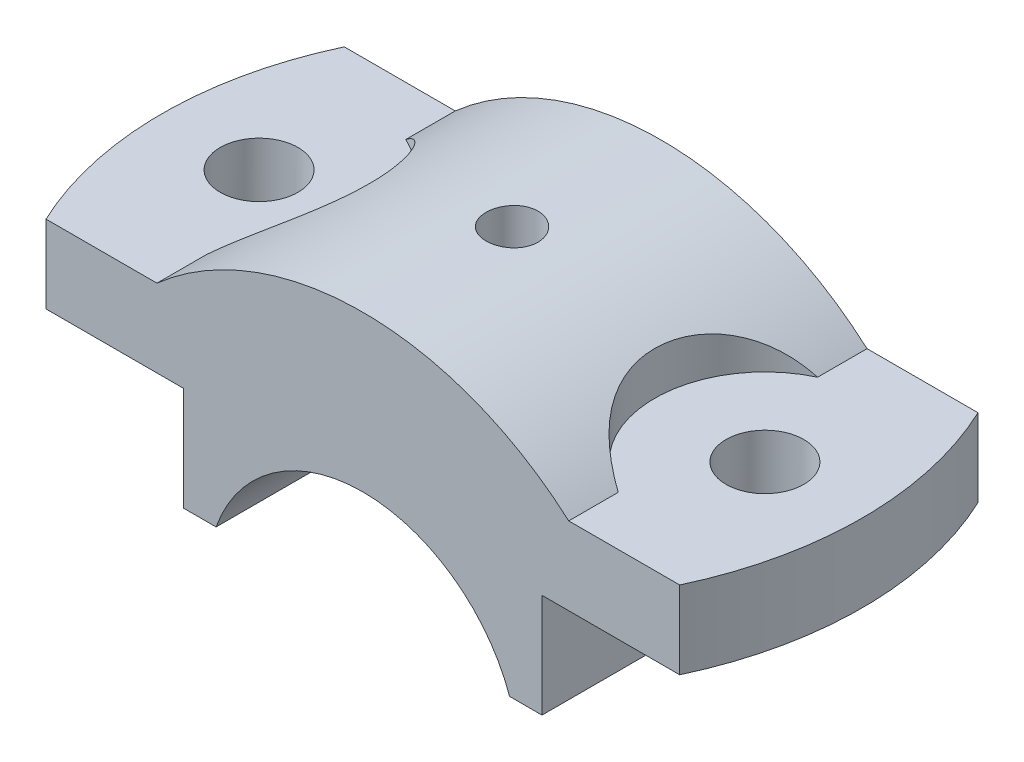
ISO-10303-21;
HEADER;
FILE_DESCRIPTION(('STEP AP214'),'2;1');
FILE_NAME('part.step','',(''),(''),'','','');
FILE_SCHEMA(('AUTOMOTIVE_DESIGN { 1 0 10303 214 1 1 1 1 }'));
ENDSEC;
DATA;
#1=APPLICATION_CONTEXT('core data for automotive mechanical design processes');
#2=APPLICATION_PROTOCOL_DEFINITION('international standard','automotive_design',2000,#1);
#3=PRODUCT_CONTEXT('',#1,'mechanical');
#4=PRODUCT('Part','Part','',(#3));
#5=PRODUCT_RELATED_PRODUCT_CATEGORY('part','',(#4));
#6=PRODUCT_DEFINITION_FORMATION('','',#4);
#7=PRODUCT_DEFINITION_CONTEXT('part definition',#1,'design');
#8=PRODUCT_DEFINITION('design','',#6,#7);
#9=PRODUCT_DEFINITION_SHAPE('','',#8);
#10=(LENGTH_UNIT() NAMED_UNIT(*) SI_UNIT(.MILLI.,.METRE.));
#11=(NAMED_UNIT(*) PLANE_ANGLE_UNIT() SI_UNIT($,.RADIAN.));
#12=(NAMED_UNIT(*) SI_UNIT($,.STERADIAN.) SOLID_ANGLE_UNIT());
#13=UNCERTAINTY_MEASURE_WITH_UNIT(LENGTH_MEASURE(1.E-05),#10,'distance_accuracy_value','');
#14=(GEOMETRIC_REPRESENTATION_CONTEXT(3) GLOBAL_UNCERTAINTY_ASSIGNED_CONTEXT((#13)) GLOBAL_UNIT_ASSIGNED_CONTEXT((#10,
#11,#12)) REPRESENTATION_CONTEXT('',''));
#15=CARTESIAN_POINT('',(0.,0.,0.));
#16=DIRECTION('',(0.,0.,1.));
#17=DIRECTION('',(1.,0.,0.));
#18=AXIS2_PLACEMENT_3D('',#15,#16,#17);
#19=CARTESIAN_POINT('',(27.6274169979695,24.,23.));
#20=DIRECTION('',(0.,1.,0.));
#21=DIRECTION('',(-1.,0.,0.));
#22=AXIS2_PLACEMENT_3D('',#19,#20,#21);
#23=PLANE('',#22);
#24=CARTESIAN_POINT('',(39.,24.,0.));
#25=DIRECTION('',(0.,1.,0.));
#26=DIRECTION('',(-1.,0.,0.));
#27=AXIS2_PLACEMENT_3D('',#24,#25,#26);
#28=CIRCLE('',#27,5.99999999999999);
#29=CARTESIAN_POINT('',(33.,24.,0.));
#30=VERTEX_POINT('',#29);
#31=EDGE_CURVE('E177',#30,#30,#28,.T.);
#32=ORIENTED_EDGE('',*,*,#31,.T.);
#33=EDGE_LOOP('',(#32));
#34=FACE_BOUND('',#33,.T.);
#35=CARTESIAN_POINT('',(0.,24.,0.));
#36=DIRECTION('',(0.,1.,0.));
#37=DIRECTION('',(-1.,0.,0.));
#38=AXIS2_PLACEMENT_3D('',#35,#36,#37);
#39=CIRCLE('',#38,54.);
#40=CARTESIAN_POINT('',(48.8569340012244,24.,23.));
#41=VERTEX_POINT('',#40);
#42=CARTESIAN_POINT('',(48.8569340012244,24.,-23.));
#43=VERTEX_POINT('',#42);
#44=EDGE_CURVE('E57',#41,#43,#39,.T.);
#45=ORIENTED_EDGE('',*,*,#44,.F.);
#46=DIRECTION('',(1.,0.,0.));
#47=VECTOR('',#46,1.);
#48=CARTESIAN_POINT('',(27.6274169979695,24.,23.));
#49=LINE('',#48,#47);
#50=CARTESIAN_POINT('',(27.6274169979695,24.,23.));
#51=VERTEX_POINT('',#50);
#52=EDGE_CURVE('E314',#51,#41,#49,.T.);
#53=ORIENTED_EDGE('',*,*,#52,.F.);
#54=DIRECTION('',(0.,0.,-1.));
#55=VECTOR('',#54,1.);
#56=CARTESIAN_POINT('',(27.6274169979695,24.,23.));
#57=LINE('',#56,#55);
#58=CARTESIAN_POINT('',(27.6274169979695,24.,-23.));
#59=VERTEX_POINT('',#58);
#60=EDGE_CURVE('E213',#51,#59,#57,.T.);
#61=ORIENTED_EDGE('',*,*,#60,.T.);
#62=DIRECTION('',(1.,0.,0.));
#63=VECTOR('',#62,1.);
#64=CARTESIAN_POINT('',(27.6274169979695,24.,-23.));
#65=LINE('',#64,#63);
#66=EDGE_CURVE('E182',#59,#43,#65,.T.);
#67=ORIENTED_EDGE('',*,*,#66,.T.);
#68=EDGE_LOOP('',(#45,#53,#61,#67));
#69=FACE_BOUND('',#68,.T.);
#70=ADVANCED_FACE('F37',(#34,#69),#23,.F.);
#71=CARTESIAN_POINT('',(54.,36.,23.));
#72=DIRECTION('',(0.,-1.,0.));
#73=DIRECTION('',(0.,0.,-1.));
#74=AXIS2_PLACEMENT_3D('',#71,#72,#73);
#75=PLANE('',#74);
#76=CARTESIAN_POINT('',(39.,36.,0.));
#77=DIRECTION('',(0.,1.,0.));
#78=DIRECTION('',(0.,0.,1.));
#79=AXIS2_PLACEMENT_3D('',#76,#77,#78);
#80=CIRCLE('',#79,6.);
#81=CARTESIAN_POINT('',(39.,36.,6.));
#82=VERTEX_POINT('',#81);
#83=EDGE_CURVE('E322',#82,#82,#80,.T.);
#84=ORIENTED_EDGE('',*,*,#83,.F.);
#85=EDGE_LOOP('',(#84));
#86=FACE_BOUND('',#85,.T.);
#87=CARTESIAN_POINT('',(0.,36.,0.));
#88=DIRECTION('',(0.,1.,0.));
#89=DIRECTION('',(0.,0.,1.));
#90=AXIS2_PLACEMENT_3D('',#87,#88,#89);
#91=CIRCLE('',#90,54.);
#92=CARTESIAN_POINT('',(48.8569340012244,36.,23.));
#93=VERTEX_POINT('',#92);
#94=CARTESIAN_POINT('',(48.8569340012244,36.,-23.));
#95=VERTEX_POINT('',#94);
#96=EDGE_CURVE('E150',#93,#95,#91,.T.);
#97=ORIENTED_EDGE('',*,*,#96,.T.);
#98=DIRECTION('',(-1.,0.,0.));
#99=VECTOR('',#98,1.);
#100=CARTESIAN_POINT('',(54.,36.,-23.));
#101=LINE('',#100,#99);
#102=CARTESIAN_POINT('',(31.7490157327751,36.,-23.));
#103=VERTEX_POINT('',#102);
#104=EDGE_CURVE('E187',#95,#103,#101,.T.);
#105=ORIENTED_EDGE('',*,*,#104,.T.);
#106=DIRECTION('',(0.,0.,-1.));
#107=VECTOR('',#106,1.);
#108=CARTESIAN_POINT('',(31.7490157327751,36.,23.));
#109=LINE('',#108,#107);
#110=CARTESIAN_POINT('',(31.7490157327751,36.,-15.3760601961769));
#111=VERTEX_POINT('',#110);
#112=EDGE_CURVE('E208',#111,#103,#109,.T.);
#113=ORIENTED_EDGE('',*,*,#112,.F.);
#114=CARTESIAN_POINT('',(39.,36.,0.));
#115=DIRECTION('',(0.,-1.,0.));
#116=DIRECTION('',(0.,0.,-1.));
#117=AXIS2_PLACEMENT_3D('',#114,#115,#116);
#118=CIRCLE('',#117,17.);
#119=CARTESIAN_POINT('',(31.7490157327751,36.,15.3760601961769));
#120=VERTEX_POINT('',#119);
#121=EDGE_CURVE('E332',#120,#111,#118,.T.);
#122=ORIENTED_EDGE('',*,*,#121,.F.);
#123=CARTESIAN_POINT('',(31.7490157327751,36.,23.));
#124=VERTEX_POINT('',#123);
#125=EDGE_CURVE('E214',#124,#120,#109,.T.);
#126=ORIENTED_EDGE('',*,*,#125,.F.);
#127=DIRECTION('',(-1.,0.,0.));
#128=VECTOR('',#127,1.);
#129=CARTESIAN_POINT('',(54.,36.,23.));
#130=LINE('',#129,#128);
#131=EDGE_CURVE('E170',#93,#124,#130,.T.);
#132=ORIENTED_EDGE('',*,*,#131,.F.);
#133=EDGE_LOOP('',(#97,#105,#113,#122,#126,#132));
#134=FACE_BOUND('',#133,.T.);
#135=ADVANCED_FACE('F276',(#86,#134),#75,.F.);
#136=CARTESIAN_POINT('',(-54.,36.,23.));
#137=DIRECTION('',(0.,-1.,0.));
#138=DIRECTION('',(0.,0.,-1.));
#139=AXIS2_PLACEMENT_3D('',#136,#137,#138);
#140=PLANE('',#139);
#141=CARTESIAN_POINT('',(-39.,36.,0.));
#142=DIRECTION('',(0.,1.,0.));
#143=DIRECTION('',(0.,0.,1.));
#144=AXIS2_PLACEMENT_3D('',#141,#142,#143);
#145=CIRCLE('',#144,6.);
#146=CARTESIAN_POINT('',(-39.,36.,6.));
#147=VERTEX_POINT('',#146);
#148=EDGE_CURVE('E333',#147,#147,#145,.T.);
#149=ORIENTED_EDGE('',*,*,#148,.F.);
#150=EDGE_LOOP('',(#149));
#151=FACE_BOUND('',#150,.T.);
#152=CARTESIAN_POINT('',(0.,36.,0.));
#153=DIRECTION('',(0.,1.,0.));
#154=DIRECTION('',(0.,0.,-1.));
#155=AXIS2_PLACEMENT_3D('',#152,#153,#154);
#156=CIRCLE('',#155,54.);
#157=CARTESIAN_POINT('',(-48.8569340012244,36.,-23.));
#158=VERTEX_POINT('',#157);
#159=CARTESIAN_POINT('',(-48.8569340012244,36.,23.));
#160=VERTEX_POINT('',#159);
#161=EDGE_CURVE('E65',#158,#160,#156,.T.);
#162=ORIENTED_EDGE('',*,*,#161,.T.);
#163=DIRECTION('',(-1.,0.,0.));
#164=VECTOR('',#163,1.);
#165=CARTESIAN_POINT('',(-54.,36.,23.));
#166=LINE('',#165,#164);
#167=CARTESIAN_POINT('',(-31.7490157327751,36.,23.));
#168=VERTEX_POINT('',#167);
#169=EDGE_CURVE('E143',#168,#160,#166,.T.);
#170=ORIENTED_EDGE('',*,*,#169,.F.);
#171=DIRECTION('',(0.,0.,-1.));
#172=VECTOR('',#171,1.);
#173=CARTESIAN_POINT('',(-31.7490157327751,36.,23.));
#174=LINE('',#173,#172);
#175=CARTESIAN_POINT('',(-31.7490157327751,36.,15.3760601961769));
#176=VERTEX_POINT('',#175);
#177=EDGE_CURVE('E206',#168,#176,#174,.T.);
#178=ORIENTED_EDGE('',*,*,#177,.T.);
#179=CARTESIAN_POINT('',(-39.,36.,0.));
#180=DIRECTION('',(0.,-1.,0.));
#181=DIRECTION('',(0.,0.,-1.));
#182=AXIS2_PLACEMENT_3D('',#179,#180,#181);
#183=CIRCLE('',#182,17.);
#184=CARTESIAN_POINT('',(-31.7490157327751,36.,-15.3760601961769));
#185=VERTEX_POINT('',#184);
#186=EDGE_CURVE('E337',#185,#176,#183,.T.);
#187=ORIENTED_EDGE('',*,*,#186,.F.);
#188=CARTESIAN_POINT('',(-31.7490157327751,36.,-23.));
#189=VERTEX_POINT('',#188);
#190=EDGE_CURVE('E210',#185,#189,#174,.T.);
#191=ORIENTED_EDGE('',*,*,#190,.T.);
#192=DIRECTION('',(-1.,0.,0.));
#193=VECTOR('',#192,1.);
#194=CARTESIAN_POINT('',(-54.,36.,-23.));
#195=LINE('',#194,#193);
#196=EDGE_CURVE('E146',#189,#158,#195,.T.);
#197=ORIENTED_EDGE('',*,*,#196,.T.);
#198=EDGE_LOOP('',(#162,#170,#178,#187,#191,#197));
#199=FACE_BOUND('',#198,.T.);
#200=ADVANCED_FACE('F145',(#151,#199),#140,.F.);
#201=CARTESIAN_POINT('',(-27.6274169979695,24.,23.));
#202=DIRECTION('',(0.,1.,0.));
#203=DIRECTION('',(-1.,0.,0.));
#204=AXIS2_PLACEMENT_3D('',#201,#202,#203);
#205=PLANE('',#204);
#206=CARTESIAN_POINT('',(-39.,24.,0.));
#207=DIRECTION('',(0.,1.,0.));
#208=DIRECTION('',(-1.,0.,0.));
#209=AXIS2_PLACEMENT_3D('',#206,#207,#208);
#210=CIRCLE('',#209,5.99999999999999);
#211=CARTESIAN_POINT('',(-45.,24.,0.));
#212=VERTEX_POINT('',#211);
#213=EDGE_CURVE('E330',#212,#212,#210,.T.);
#214=ORIENTED_EDGE('',*,*,#213,.T.);
#215=EDGE_LOOP('',(#214));
#216=FACE_BOUND('',#215,.T.);
#217=DIRECTION('',(1.,0.,0.));
#218=VECTOR('',#217,1.);
#219=CARTESIAN_POINT('',(-27.6274169979695,24.,23.));
#220=LINE('',#219,#218);
#221=CARTESIAN_POINT('',(-48.8569340012244,24.,23.));
#222=VERTEX_POINT('',#221);
#223=CARTESIAN_POINT('',(-27.6274169979695,24.,23.));
#224=VERTEX_POINT('',#223);
#225=EDGE_CURVE('E161',#222,#224,#220,.T.);
#226=ORIENTED_EDGE('',*,*,#225,.F.);
#227=CARTESIAN_POINT('',(0.,24.,0.));
#228=DIRECTION('',(0.,1.,0.));
#229=DIRECTION('',(-1.,0.,0.));
#230=AXIS2_PLACEMENT_3D('',#227,#228,#229);
#231=CIRCLE('',#230,54.);
#232=CARTESIAN_POINT('',(-48.8569340012244,24.,-23.));
#233=VERTEX_POINT('',#232);
#234=EDGE_CURVE('E151',#233,#222,#231,.T.);
#235=ORIENTED_EDGE('',*,*,#234,.F.);
#236=DIRECTION('',(1.,0.,0.));
#237=VECTOR('',#236,1.);
#238=CARTESIAN_POINT('',(-27.6274169979695,24.,-23.));
#239=LINE('',#238,#237);
#240=CARTESIAN_POINT('',(-27.6274169979695,24.,-23.));
#241=VERTEX_POINT('',#240);
#242=EDGE_CURVE('E191',#233,#241,#239,.T.);
#243=ORIENTED_EDGE('',*,*,#242,.T.);
#244=DIRECTION('',(0.,0.,-1.));
#245=VECTOR('',#244,1.);
#246=CARTESIAN_POINT('',(-27.6274169979695,24.,23.));
#247=LINE('',#246,#245);
#248=EDGE_CURVE('E202',#224,#241,#247,.T.);
#249=ORIENTED_EDGE('',*,*,#248,.F.);
#250=EDGE_LOOP('',(#226,#235,#243,#249));
#251=FACE_BOUND('',#250,.T.);
#252=ADVANCED_FACE('F265',(#216,#251),#205,.F.);
#253=CARTESIAN_POINT('',(0.,0.,23.));
#254=DIRECTION('',(0.,0.,-1.));
#255=DIRECTION('',(-1.,0.,0.));
#256=AXIS2_PLACEMENT_3D('',#253,#254,#255);
#257=PLANE('',#256);
#258=CARTESIAN_POINT('',(0.,0.,23.));
#259=DIRECTION('',(0.,0.,1.));
#260=DIRECTION('',(-1.,0.,0.));
#261=AXIS2_PLACEMENT_3D('',#258,#259,#260);
#262=CIRCLE('',#261,48.);
#263=EDGE_CURVE('E163',#124,#168,#262,.T.);
#264=ORIENTED_EDGE('',*,*,#263,.T.);
#265=ORIENTED_EDGE('',*,*,#169,.T.);
#266=DIRECTION('',(0.,1.,0.));
#267=VECTOR('',#266,1.);
#268=CARTESIAN_POINT('',(-48.8569340012244,7.99999999999999,23.));
#269=LINE('',#268,#267);
#270=EDGE_CURVE('E152',#222,#160,#269,.T.);
#271=ORIENTED_EDGE('',*,*,#270,.F.);
#272=ORIENTED_EDGE('',*,*,#225,.T.);
#273=DIRECTION('',(0.,-1.,0.));
#274=VECTOR('',#273,1.);
#275=CARTESIAN_POINT('',(-27.6274169979695,7.99999999999999,23.));
#276=LINE('',#275,#274);
#277=CARTESIAN_POINT('',(-27.6274169979695,7.99999999999999,23.));
#278=VERTEX_POINT('',#277);
#279=EDGE_CURVE('E164',#224,#278,#276,.T.);
#280=ORIENTED_EDGE('',*,*,#279,.T.);
#281=DIRECTION('',(1.,0.,0.));
#282=VECTOR('',#281,1.);
#283=CARTESIAN_POINT('',(-22.6274169979695,8.,23.));
#284=LINE('',#283,#282);
#285=CARTESIAN_POINT('',(-22.6274169979695,8.,23.));
#286=VERTEX_POINT('',#285);
#287=EDGE_CURVE('E175',#278,#286,#284,.T.);
#288=ORIENTED_EDGE('',*,*,#287,.T.);
#289=CARTESIAN_POINT('',(0.,0.,23.));
#290=DIRECTION('',(0.,0.,-1.));
#291=DIRECTION('',(-1.,0.,0.));
#292=AXIS2_PLACEMENT_3D('',#289,#290,#291);
#293=CIRCLE('',#292,24.);
#294=CARTESIAN_POINT('',(22.6274169979695,8.,23.));
#295=VERTEX_POINT('',#294);
#296=EDGE_CURVE('E200',#286,#295,#293,.T.);
#297=ORIENTED_EDGE('',*,*,#296,.T.);
#298=DIRECTION('',(1.,0.,0.));
#299=VECTOR('',#298,1.);
#300=CARTESIAN_POINT('',(22.6274169979695,8.,23.));
#301=LINE('',#300,#299);
#302=CARTESIAN_POINT('',(27.6274169979695,7.99999999999999,23.));
#303=VERTEX_POINT('',#302);
#304=EDGE_CURVE('E319',#295,#303,#301,.T.);
#305=ORIENTED_EDGE('',*,*,#304,.T.);
#306=DIRECTION('',(0.,1.,0.));
#307=VECTOR('',#306,1.);
#308=CARTESIAN_POINT('',(27.6274169979695,7.99999999999999,23.));
#309=LINE('',#308,#307);
#310=EDGE_CURVE('E307',#303,#51,#309,.T.);
#311=ORIENTED_EDGE('',*,*,#310,.T.);
#312=ORIENTED_EDGE('',*,*,#52,.T.);
#313=DIRECTION('',(0.,1.,0.));
#314=VECTOR('',#313,1.);
#315=CARTESIAN_POINT('',(48.8569340012244,7.99999999999999,23.));
#316=LINE('',#315,#314);
#317=EDGE_CURVE('E160',#41,#93,#316,.T.);
#318=ORIENTED_EDGE('',*,*,#317,.T.);
#319=ORIENTED_EDGE('',*,*,#131,.T.);
#320=EDGE_LOOP('',(#264,#265,#271,#272,#280,#288,#297,#305,#311,#312,#318,#319));
#321=FACE_BOUND('',#320,.T.);
#322=ADVANCED_FACE('F157',(#321),#257,.F.);
#323=CARTESIAN_POINT('',(0.,0.,-23.));
#324=DIRECTION('',(0.,0.,-1.));
#325=DIRECTION('',(-1.,0.,0.));
#326=AXIS2_PLACEMENT_3D('',#323,#324,#325);
#327=PLANE('',#326);
#328=CARTESIAN_POINT('',(0.,0.,-23.));
#329=DIRECTION('',(0.,0.,1.));
#330=DIRECTION('',(-1.,0.,0.));
#331=AXIS2_PLACEMENT_3D('',#328,#329,#330);
#332=CIRCLE('',#331,48.);
#333=EDGE_CURVE('E189',#103,#189,#332,.T.);
#334=ORIENTED_EDGE('',*,*,#333,.F.);
#335=ORIENTED_EDGE('',*,*,#104,.F.);
#336=DIRECTION('',(0.,1.,0.));
#337=VECTOR('',#336,1.);
#338=CARTESIAN_POINT('',(48.8569340012244,7.99999999999999,-23.));
#339=LINE('',#338,#337);
#340=EDGE_CURVE('E12',#95,#43,#339,.F.);
#341=ORIENTED_EDGE('',*,*,#340,.T.);
#342=ORIENTED_EDGE('',*,*,#66,.F.);
#343=DIRECTION('',(0.,1.,0.));
#344=VECTOR('',#343,1.);
#345=CARTESIAN_POINT('',(27.6274169979695,7.99999999999999,-23.));
#346=LINE('',#345,#344);
#347=CARTESIAN_POINT('',(27.6274169979695,7.99999999999999,-23.));
#348=VERTEX_POINT('',#347);
#349=EDGE_CURVE('E181',#348,#59,#346,.T.);
#350=ORIENTED_EDGE('',*,*,#349,.F.);
#351=DIRECTION('',(1.,0.,0.));
#352=VECTOR('',#351,1.);
#353=CARTESIAN_POINT('',(22.6274169979695,8.,-23.));
#354=LINE('',#353,#352);
#355=CARTESIAN_POINT('',(22.6274169979695,8.,-23.));
#356=VERTEX_POINT('',#355);
#357=EDGE_CURVE('E178',#356,#348,#354,.T.);
#358=ORIENTED_EDGE('',*,*,#357,.F.);
#359=CARTESIAN_POINT('',(0.,0.,-23.));
#360=DIRECTION('',(0.,0.,-1.));
#361=DIRECTION('',(-1.,0.,0.));
#362=AXIS2_PLACEMENT_3D('',#359,#360,#361);
#363=CIRCLE('',#362,24.);
#364=CARTESIAN_POINT('',(-22.6274169979695,8.,-23.));
#365=VERTEX_POINT('',#364);
#366=EDGE_CURVE('E174',#365,#356,#363,.T.);
#367=ORIENTED_EDGE('',*,*,#366,.F.);
#368=DIRECTION('',(1.,0.,0.));
#369=VECTOR('',#368,1.);
#370=CARTESIAN_POINT('',(-22.6274169979695,8.,-23.));
#371=LINE('',#370,#369);
#372=CARTESIAN_POINT('',(-27.6274169979695,7.99999999999999,-23.));
#373=VERTEX_POINT('',#372);
#374=EDGE_CURVE('E197',#373,#365,#371,.T.);
#375=ORIENTED_EDGE('',*,*,#374,.F.);
#376=DIRECTION('',(0.,-1.,0.));
#377=VECTOR('',#376,1.);
#378=CARTESIAN_POINT('',(-27.6274169979695,7.99999999999999,-23.));
#379=LINE('',#378,#377);
#380=EDGE_CURVE('E193',#241,#373,#379,.T.);
#381=ORIENTED_EDGE('',*,*,#380,.F.);
#382=ORIENTED_EDGE('',*,*,#242,.F.);
#383=DIRECTION('',(0.,1.,0.));
#384=VECTOR('',#383,1.);
#385=CARTESIAN_POINT('',(-48.8569340012244,7.99999999999999,-23.));
#386=LINE('',#385,#384);
#387=EDGE_CURVE('E47',#233,#158,#386,.T.);
#388=ORIENTED_EDGE('',*,*,#387,.T.);
#389=ORIENTED_EDGE('',*,*,#196,.F.);
#390=EDGE_LOOP('',(#334,#335,#341,#342,#350,#358,#367,#375,#381,#382,#388,#389));
#391=FACE_BOUND('',#390,.T.);
#392=ADVANCED_FACE('F264',(#391),#327,.T.);
#393=CARTESIAN_POINT('',(0.,0.,23.));
#394=DIRECTION('',(0.,0.,-1.));
#395=DIRECTION('',(-1.,0.,0.));
#396=AXIS2_PLACEMENT_3D('',#393,#394,#395);
#397=CYLINDRICAL_SURFACE('',#396,24.);
#398=CARTESIAN_POINT('',(0.,24.,3.));
#399=CARTESIAN_POINT('',(0.167809314666914,23.9999976587571,2.99999287087714));
#400=CARTESIAN_POINT('',(0.335723489163297,23.9982214146588,2.98587254499686));
#401=CARTESIAN_POINT('',(0.666879362507704,23.9913064813363,2.92976669451505));
#402=CARTESIAN_POINT('',(0.830115996748494,23.9861642812971,2.88775207449193));
#403=CARTESIAN_POINT('',(1.14707468977566,23.9730967325329,2.7771148273031));
#404=CARTESIAN_POINT('',(1.30080307217537,23.9651732574665,2.70851010982817));
#405=CARTESIAN_POINT('',(1.59453536987164,23.9474244105372,2.54667925923625));
#406=CARTESIAN_POINT('',(1.73454163386764,23.9375993650094,2.45345734976314));
#407=CARTESIAN_POINT('',(1.99765538031758,23.9170838556759,2.24448966019249));
#408=CARTESIAN_POINT('',(2.12067643792455,23.906389376309,2.12863544478451));
#409=CARTESIAN_POINT('',(2.34558335226899,23.885372712117,1.87792461175603));
#410=CARTESIAN_POINT('',(2.4474681316707,23.8750505462912,1.7430670261041));
#411=CARTESIAN_POINT('',(2.62753219354073,23.855907667435,1.4576160269212));
#412=CARTESIAN_POINT('',(2.70563051512929,23.8470921261349,1.30697116611847));
#413=CARTESIAN_POINT('',(2.83538769189014,23.8320135414922,0.994575537663167));
#414=CARTESIAN_POINT('',(2.88704754967826,23.8257504013576,0.832825191423583));
#415=CARTESIAN_POINT('',(2.96219877602972,23.8165240752434,0.503706965295881));
#416=CARTESIAN_POINT('',(2.98583605767804,23.8135438012409,0.336372890754967));
#417=CARTESIAN_POINT('',(3.00472265946868,23.8111683377135,8.84838337999864E-05));
#418=CARTESIAN_POINT('',(2.9999731212029,23.8117730040181,-0.168861783277549));
#419=CARTESIAN_POINT('',(2.96234068373748,23.816483464437,-0.502565792698538));
#420=CARTESIAN_POINT('',(2.92961851558164,23.8205692555239,-0.667337983440315));
#421=CARTESIAN_POINT('',(2.83722045981846,23.8317503970915,-0.989034025462784));
#422=CARTESIAN_POINT('',(2.77754402610228,23.8388458085487,-1.14595771765685));
#423=CARTESIAN_POINT('',(2.63275867189398,23.8552693903758,-1.44800159882602));
#424=CARTESIAN_POINT('',(2.54757990444916,23.8646036785373,-1.59308796029878));
#425=CARTESIAN_POINT('',(2.3542577633483,23.8844485371672,-1.8669680332959));
#426=CARTESIAN_POINT('',(2.24611333929693,23.8949591614279,-1.99576099916842));
#427=CARTESIAN_POINT('',(2.00903893290454,23.9160613186851,-2.23433125286729));
#428=CARTESIAN_POINT('',(1.87997040940802,23.9266529086427,-2.34397091011918));
#429=CARTESIAN_POINT('',(1.60518860293671,23.9466555906702,-2.54005065603666));
#430=CARTESIAN_POINT('',(1.4594752815819,23.9560666800181,-2.6264906912064));
#431=CARTESIAN_POINT('',(1.15543400563618,23.972653826623,-2.7737175845567));
#432=CARTESIAN_POINT('',(0.997101834405261,23.9798291328184,-2.83449582465747));
#433=CARTESIAN_POINT('',(0.672369528517268,23.9911294293607,-2.9285645922279));
#434=CARTESIAN_POINT('',(0.505969771956801,23.9952545625104,-2.96185640656446));
#435=CARTESIAN_POINT('',(0.171015796696197,23.9999711569291,-2.99982890911266));
#436=CARTESIAN_POINT('',(0.00248338823832908,24.0005860337116,-3.00469919083688));
#437=CARTESIAN_POINT('',(-0.332995243796995,23.9982760560652,-2.98619071913286));
#438=CARTESIAN_POINT('',(-0.499941501077647,23.9953512770186,-2.96281256729809));
#439=CARTESIAN_POINT('',(-0.826949409265826,23.9863052250803,-2.88862834947074));
#440=CARTESIAN_POINT('',(-0.987031884509646,23.9801944897664,-2.83791268391684));
#441=CARTESIAN_POINT('',(-1.29641958583009,23.9654606772024,-2.7105870577045));
#442=CARTESIAN_POINT('',(-1.44572444575838,23.9568375146475,-2.63397621781029));
#443=CARTESIAN_POINT('',(-1.73016542482491,23.9379818749213,-2.45657623499105));
#444=CARTESIAN_POINT('',(-1.86522451193258,23.9277413285101,-2.35566445223324));
#445=CARTESIAN_POINT('',(-2.11655638755158,23.9068217079079,-2.13270060295896));
#446=CARTESIAN_POINT('',(-2.23282843000423,23.8961426163228,-2.01064769729881));
#447=CARTESIAN_POINT('',(-2.44395835058162,23.875477265551,-1.74803109989143));
#448=CARTESIAN_POINT('',(-2.53869055268152,23.8654952966559,-1.60736598442753));
#449=CARTESIAN_POINT('',(-2.70318346733221,23.8474249324458,-1.31201010617435));
#450=CARTESIAN_POINT('',(-2.77294468047404,23.8393364991723,-1.15731962462818));
#451=CARTESIAN_POINT('',(-2.88531189463985,23.8259982047159,-0.838709617022865));
#452=CARTESIAN_POINT('',(-2.92798875294853,23.8207409422175,-0.674815403942435));
#453=CARTESIAN_POINT('',(-2.98520399264142,23.8136389908895,-0.342117019463202));
#454=CARTESIAN_POINT('',(-2.99974368304292,23.8117941433053,-0.173313076849199));
#455=CARTESIAN_POINT('',(-3.0002478433018,23.8117305237895,0.163162715045614));
#456=CARTESIAN_POINT('',(-2.98640975723913,23.8134866970234,0.330834297998265));
#457=CARTESIAN_POINT('',(-2.93096928581919,23.8203733744464,0.661448555214093));
#458=CARTESIAN_POINT('',(-2.88936689748692,23.825503878997,0.824391228970554));
#459=CARTESIAN_POINT('',(-2.77964048842759,23.8385533892946,1.14089634811968));
#460=CARTESIAN_POINT('',(-2.71152597716512,23.8464713951134,1.29446213402618));
#461=CARTESIAN_POINT('',(-2.55072828258037,23.8642053989378,1.58801598485798));
#462=CARTESIAN_POINT('',(-2.45804479141151,23.874021420725,1.72800387962379));
#463=CARTESIAN_POINT('',(-2.25000759751901,23.8945272570268,1.99143747040857));
#464=CARTESIAN_POINT('',(-2.13450675092995,23.9052224650084,2.11476655314597));
#465=CARTESIAN_POINT('',(-1.88442027236206,23.9262339791148,2.34036819020157));
#466=CARTESIAN_POINT('',(-1.74983014696988,23.9365501953071,2.44263577292917));
#467=CARTESIAN_POINT('',(-1.46479874502505,23.955684679041,2.62354242852635));
#468=CARTESIAN_POINT('',(-1.3142991355154,23.9644971009396,2.70209016707911));
#469=CARTESIAN_POINT('',(-1.00221948276154,23.9795717889207,2.83268549149954));
#470=CARTESIAN_POINT('',(-0.840651697044284,23.9858368244349,2.88476187162415));
#471=CARTESIAN_POINT('',(-0.56520692636151,23.993600643933,2.94847120580557));
#472=CARTESIAN_POINT('',(-0.453066796220305,23.9959887107454,2.96776673037848));
#473=CARTESIAN_POINT('',(-0.227300475854922,23.9991891759503,2.99353349483187));
#474=CARTESIAN_POINT('',(-0.113674296595233,24.0000015859616,3.00000482927916));
#475=CARTESIAN_POINT('',(0.,24.,3.));
#476=B_SPLINE_CURVE_WITH_KNOTS('',3,(#398,#399,#400,#401,#402,#403,#404,#405,#406,#407,#408,
#409,#410,#411,#412,#413,#414,#415,#416,#417,#418,#419,#420,#421,#422,#423,#424,#425,#426,#427,
#428,#429,#430,#431,#432,#433,#434,#435,#436,#437,#438,#439,#440,#441,#442,#443,#444,#445,#446,
#447,#448,#449,#450,#451,#452,#453,#454,#455,#456,#457,#458,#459,#460,#461,#462,#463,#464,#465,
#466,#467,#468,#469,#470,#471,#472,#473,#474,#475),.UNSPECIFIED.,.T.,.F.,(4,2,2,2,2,2,2,2,2,2,2,
2,2,2,2,2,2,2,2,2,2,2,2,2,2,2,2,2,2,2,2,2,2,2,2,2,2,2,4),(0.,0.503012727331497,1.00655095313211,
1.50975060981812,2.01286398709288,2.51844975842212,3.02406129360013,3.53137500382643,
4.03866947396168,4.54331070343585,5.04793163861596,5.5496723573003,6.0514232419949,
6.5545611154264,7.05772200616366,7.564361737637,8.07100263735736,8.57781354877926,
9.08460073084536,9.58800335270305,10.0913952540231,10.5931326467208,11.0948870769474,
11.5992288351411,12.1035906165011,12.6108236580909,13.1180465306585,13.6239368913711,
14.1298037161275,14.6321628144266,15.1345219665546,15.6367010964779,16.1388865189472,
16.644422852302,17.1500783816402,17.6576568364422,18.1646819842084,18.5054261182515,
18.8461677396052),.UNSPECIFIED.);
#477=CARTESIAN_POINT('',(0.,24.,3.));
#478=VERTEX_POINT('',#477);
#479=EDGE_CURVE('E344',#478,#478,#476,.T.);
#480=ORIENTED_EDGE('',*,*,#479,.T.);
#481=EDGE_LOOP('',(#480));
#482=FACE_BOUND('',#481,.T.);
#483=ORIENTED_EDGE('',*,*,#366,.T.);
#484=DIRECTION('',(0.,0.,-1.));
#485=VECTOR('',#484,1.);
#486=CARTESIAN_POINT('',(22.6274169979695,8.,23.));
#487=LINE('',#486,#485);
#488=EDGE_CURVE('E218',#295,#356,#487,.T.);
#489=ORIENTED_EDGE('',*,*,#488,.F.);
#490=ORIENTED_EDGE('',*,*,#296,.F.);
#491=DIRECTION('',(0.,0.,-1.));
#492=VECTOR('',#491,1.);
#493=CARTESIAN_POINT('',(-22.6274169979695,8.,23.));
#494=LINE('',#493,#492);
#495=EDGE_CURVE('E172',#286,#365,#494,.T.);
#496=ORIENTED_EDGE('',*,*,#495,.T.);
#497=EDGE_LOOP('',(#483,#489,#490,#496));
#498=FACE_BOUND('',#497,.T.);
#499=ADVANCED_FACE('F45',(#482,#498),#397,.F.);
#500=CARTESIAN_POINT('',(22.6274169979695,8.,23.));
#501=DIRECTION('',(0.,1.,0.));
#502=DIRECTION('',(-1.,0.,0.));
#503=AXIS2_PLACEMENT_3D('',#500,#501,#502);
#504=PLANE('',#503);
#505=ORIENTED_EDGE('',*,*,#357,.T.);
#506=DIRECTION('',(0.,0.,-1.));
#507=VECTOR('',#506,1.);
#508=CARTESIAN_POINT('',(27.6274169979695,7.99999999999999,23.));
#509=LINE('',#508,#507);
#510=EDGE_CURVE('E219',#303,#348,#509,.T.);
#511=ORIENTED_EDGE('',*,*,#510,.F.);
#512=ORIENTED_EDGE('',*,*,#304,.F.);
#513=ORIENTED_EDGE('',*,*,#488,.T.);
#514=EDGE_LOOP('',(#505,#511,#512,#513));
#515=FACE_BOUND('',#514,.T.);
#516=ADVANCED_FACE('F294',(#515),#504,.F.);
#517=CARTESIAN_POINT('',(27.6274169979695,7.99999999999999,23.));
#518=DIRECTION('',(-1.,0.,0.));
#519=DIRECTION('',(0.,-1.,0.));
#520=AXIS2_PLACEMENT_3D('',#517,#518,#519);
#521=PLANE('',#520);
#522=ORIENTED_EDGE('',*,*,#349,.T.);
#523=ORIENTED_EDGE('',*,*,#60,.F.);
#524=ORIENTED_EDGE('',*,*,#310,.F.);
#525=ORIENTED_EDGE('',*,*,#510,.T.);
#526=EDGE_LOOP('',(#522,#523,#524,#525));
#527=FACE_BOUND('',#526,.T.);
#528=ADVANCED_FACE('F291',(#527),#521,.F.);
#529=CARTESIAN_POINT('',(0.,0.,23.));
#530=DIRECTION('',(0.,0.,-1.));
#531=DIRECTION('',(-1.,0.,0.));
#532=AXIS2_PLACEMENT_3D('',#529,#530,#531);
#533=CYLINDRICAL_SURFACE('',#532,48.);
#534=CARTESIAN_POINT('',(0.,48.,4.));
#535=CARTESIAN_POINT('',(-0.224264359684817,47.9999978164606,3.99999020469488));
#536=CARTESIAN_POINT('',(-0.448681388720903,47.9984115417359,3.98107612075582));
#537=CARTESIAN_POINT('',(-0.891306282801559,47.99223609313,3.90590259257969));
#538=CARTESIAN_POINT('',(-1.10950682090092,47.9876435172678,3.84960083878039));
#539=CARTESIAN_POINT('',(-1.53322409005704,47.9759744498442,3.70129138476253));
#540=CARTESIAN_POINT('',(-1.73874792169846,47.9688993639394,3.60930388756073));
#541=CARTESIAN_POINT('',(-2.13138893366431,47.9530587097885,3.39227027251202));
#542=CARTESIAN_POINT('',(-2.31851003954156,47.9442935032543,3.26723122608997));
#543=CARTESIAN_POINT('',(-2.66955999986236,47.9260311946685,2.98729973357602));
#544=CARTESIAN_POINT('',(-2.83343548966465,47.9165324834631,2.83234046425725));
#545=CARTESIAN_POINT('',(-3.13288453414622,47.8978872321267,2.49710841660026));
#546=CARTESIAN_POINT('',(-3.26845684548602,47.8887407074816,2.31683452678951));
#547=CARTESIAN_POINT('',(-3.50763168956092,47.8718181064497,1.93576753160388));
#548=CARTESIAN_POINT('',(-3.61118733180617,47.8640440472037,1.73494489838891));
#549=CARTESIAN_POINT('',(-3.78308973509538,47.8507649779309,1.31868681777607));
#550=CARTESIAN_POINT('',(-3.85143711804967,47.8452599278253,1.10325162856699));
#551=CARTESIAN_POINT('',(-3.95082811927428,47.8371556826529,0.664418432475287));
#552=CARTESIAN_POINT('',(-3.9819586615591,47.8345497174488,0.441040240029589));
#553=CARTESIAN_POINT('',(-4.00630083206171,47.832517292859,-0.00778481578146548));
#554=CARTESIAN_POINT('',(-3.99951317191816,47.8330907738024,-0.233231640244013));
#555=CARTESIAN_POINT('',(-3.94828345685939,47.8373462944655,-0.679198662042087));
#556=CARTESIAN_POINT('',(-3.90393587215223,47.8410205351141,-0.899729796305651));
#557=CARTESIAN_POINT('',(-3.77899194153176,47.8510513427746,-1.33020746957181));
#558=CARTESIAN_POINT('',(-3.69839524158714,47.857407935984,-1.54015390517541));
#559=CARTESIAN_POINT('',(-3.50313515260813,47.8720961882741,-1.94380362351239));
#560=CARTESIAN_POINT('',(-3.38842937902877,47.8804303020386,-2.13748631035003));
#561=CARTESIAN_POINT('',(-3.12823777565339,47.8981322745552,-2.50288535527922));
#562=CARTESIAN_POINT('',(-2.98275132249016,47.9075001542413,-2.67460126838886));
#563=CARTESIAN_POINT('',(-2.66459832890545,47.9262488164658,-2.99174167712627));
#564=CARTESIAN_POINT('',(-2.4918501175623,47.9356295510027,-3.13708425651701));
#565=CARTESIAN_POINT('',(-2.124362225487,47.9533196747934,-3.39671889355421));
#566=CARTESIAN_POINT('',(-1.92962253006135,47.9616290633314,-3.51101093045423));
#567=CARTESIAN_POINT('',(-1.5236263730714,47.9762418323856,-3.70529505067482));
#568=CARTESIAN_POINT('',(-1.31236816723629,47.9825450006977,-3.78528350591262));
#569=CARTESIAN_POINT('',(-0.879356276078325,47.9924326964719,-3.90863252980531));
#570=CARTESIAN_POINT('',(-0.657602808675418,47.9960172803554,-3.95199385862105));
#571=CARTESIAN_POINT('',(-0.210605200657002,48.000056677722,-4.00075505616631));
#572=CARTESIAN_POINT('',(0.0146265164607859,48.0005208196801,-4.00626807242759));
#573=CARTESIAN_POINT('',(0.462811010013215,47.998291951148,-3.97947255749073));
#574=CARTESIAN_POINT('',(0.685763807685654,47.995598970107,-3.94716437908216));
#575=CARTESIAN_POINT('',(1.1227390248988,47.9873647136528,-3.84573736555962));
#576=CARTESIAN_POINT('',(1.33677370055889,47.9818274966968,-3.77667097589676));
#577=CARTESIAN_POINT('',(1.75021666032996,47.968526804494,-3.60374164887188));
#578=CARTESIAN_POINT('',(1.94962471313253,47.9607632940497,-3.499878161366));
#579=CARTESIAN_POINT('',(2.32866887320763,47.9438570557453,-3.26001860313457));
#580=CARTESIAN_POINT('',(2.50825740208588,47.9347111287495,-3.12394757442069));
#581=CARTESIAN_POINT('',(2.84208437937449,47.9160783455879,-2.82364377179807));
#582=CARTESIAN_POINT('',(2.99632238725753,47.9065914835011,-2.65941050860293));
#583=CARTESIAN_POINT('',(3.27545818182041,47.8883184486329,-2.30695323120664));
#584=CARTESIAN_POINT('',(3.40028213293455,47.8795340749689,-2.1186706352104));
#585=CARTESIAN_POINT('',(3.61654025135807,47.8636860697728,-1.72375094854633));
#586=CARTESIAN_POINT('',(3.70797475203986,47.8566224210606,-1.51711404116024));
#587=CARTESIAN_POINT('',(3.85473270976226,47.8450257139576,-1.09161283784305));
#588=CARTESIAN_POINT('',(3.91010136579716,47.8404894891454,-0.872764221142676));
#589=CARTESIAN_POINT('',(3.98330307964061,47.834450627634,-0.428837200502302));
#590=CARTESIAN_POINT('',(4.00113685827306,47.8329479326787,-0.203758916281619));
#591=CARTESIAN_POINT('',(3.99875425156372,47.8331471180078,0.245504504083584));
#592=CARTESIAN_POINT('',(3.97865387910956,47.8348392277228,0.469690268945753));
#593=CARTESIAN_POINT('',(3.90121545318012,47.8412166032923,0.911490134203405));
#594=CARTESIAN_POINT('',(3.84387734291051,47.8459018737118,1.12910422457536));
#595=CARTESIAN_POINT('',(3.69362044006825,47.8577350852682,1.55159105306648));
#596=CARTESIAN_POINT('',(3.60070373602613,47.8648828818476,1.75646453826275));
#597=CARTESIAN_POINT('',(3.381940235789,47.8808359950028,2.14772336229467));
#598=CARTESIAN_POINT('',(3.25609395645823,47.8896412855619,2.3341089912533));
#599=CARTESIAN_POINT('',(2.97460776848979,47.9079492679473,2.68369495605204));
#600=CARTESIAN_POINT('',(2.81888197496583,47.9174539202297,2.84682603462939));
#601=CARTESIAN_POINT('',(2.48221290236986,47.9360718003871,3.14470074081328));
#602=CARTESIAN_POINT('',(2.30126353056436,47.945184932993,3.27943748998406));
#603=CARTESIAN_POINT('',(1.91893509211766,47.962009393691,3.51687944167025));
#604=CARTESIAN_POINT('',(1.71751862508215,47.9697180809242,3.61952455462531));
#605=CARTESIAN_POINT('',(1.30038300798293,47.982834100652,3.78940721220511));
#606=CARTESIAN_POINT('',(1.0846806216546,47.9882440771303,3.85668545715242));
#607=CARTESIAN_POINT('',(0.723088192386716,47.994764309354,3.93679033000819));
#608=CARTESIAN_POINT('',(0.57952357775388,47.9967187550781,3.96046245006995));
#609=CARTESIAN_POINT('',(0.290660686004648,47.9993373063453,3.99207043870882));
#610=CARTESIAN_POINT('',(0.145362413492179,48.0000014153143,4.00000634906587));
#611=CARTESIAN_POINT('',(0.,48.,4.));
#612=B_SPLINE_CURVE_WITH_KNOTS('',3,(#534,#535,#536,#537,#538,#539,#540,#541,#542,#543,#544,
#545,#546,#547,#548,#549,#550,#551,#552,#553,#554,#555,#556,#557,#558,#559,#560,#561,#562,#563,
#564,#565,#566,#567,#568,#569,#570,#571,#572,#573,#574,#575,#576,#577,#578,#579,#580,#581,#582,
#583,#584,#585,#586,#587,#588,#589,#590,#591,#592,#593,#594,#595,#596,#597,#598,#599,#600,#601,
#602,#603,#604,#605,#606,#607,#608,#609,#610,#611),.UNSPECIFIED.,.T.,.F.,(4,2,2,2,2,2,2,2,2,2,2,
2,2,2,2,2,2,2,2,2,2,2,2,2,2,2,2,2,2,2,2,2,2,2,2,2,2,2,4),(0.,0.672262347200557,1.34528675599134,
2.01793069555582,2.69043083833673,3.36445067514306,4.03850011495727,4.71353211804366,
5.38855219711604,6.06199259326346,6.73542035050476,7.40715932441158,8.07890485907996,
8.75148862995597,9.42408602323441,10.098738037406,10.7733905023458,11.448114303618,
12.1228241013014,12.7955159722867,13.4682015685688,14.1399299612314,14.8116689744549,
15.4849869989971,16.15831672285,16.8333190596481,17.5083146567931,18.1824626896371,
18.8565977759503,19.5286745153011,20.2007522796936,20.8727905979009,21.5448183683942,
22.2188075465856,22.8929598092992,23.5683669225021,24.2429950636714,24.6787394542665,
25.1144826879498),.UNSPECIFIED.);
#613=CARTESIAN_POINT('',(0.,48.,4.));
#614=VERTEX_POINT('',#613);
#615=EDGE_CURVE('E361',#614,#614,#612,.T.);
#616=ORIENTED_EDGE('',*,*,#615,.T.);
#617=EDGE_LOOP('',(#616));
#618=FACE_BOUND('',#617,.T.);
#619=ORIENTED_EDGE('',*,*,#190,.F.);
#620=CARTESIAN_POINT('',(-31.7490157327751,36.,-15.3760601961769));
#621=CARTESIAN_POINT('',(-31.5666993606049,36.1607910344816,-15.2900831270757));
#622=CARTESIAN_POINT('',(-31.3842407385664,36.3192382806885,-15.200076432177));
#623=CARTESIAN_POINT('',(-31.0194382984914,36.6312986785064,-15.0117552307289));
#624=CARTESIAN_POINT('',(-30.83709449581,36.7849112802083,-14.9134397837671));
#625=CARTESIAN_POINT('',(-30.2906545114745,37.2384242405059,-14.6055515958542));
#626=CARTESIAN_POINT('',(-29.9273932433292,37.5307855559239,-14.3831506648985));
#627=CARTESIAN_POINT('',(-29.2055877678829,38.0952057641667,-13.9017498917579));
#628=CARTESIAN_POINT('',(-28.8470773519233,38.3671527207169,-13.6425680163447));
#629=CARTESIAN_POINT('',(-28.1414563178619,38.8876660950044,-13.087906778826));
#630=CARTESIAN_POINT('',(-27.7943424142725,39.1362392903486,-12.7924379963692));
#631=CARTESIAN_POINT('',(-27.1144372728569,39.6103537782901,-12.1634340928703));
#632=CARTESIAN_POINT('',(-26.7817440960143,39.8357484531289,-11.8296819039898));
#633=CARTESIAN_POINT('',(-26.1381758530123,40.2609560521935,-11.1265718110928));
#634=CARTESIAN_POINT('',(-25.8273031949563,40.4607661549158,-10.7572099878546));
#635=CARTESIAN_POINT('',(-25.2335249148575,40.8337098769773,-9.98600624775001));
#636=CARTESIAN_POINT('',(-24.9505424988563,41.0069175240425,-9.58425938846313));
#637=CARTESIAN_POINT('',(-24.4165226257608,41.3271148139075,-8.75027197863382));
#638=CARTESIAN_POINT('',(-24.165480267083,41.4741084809499,-8.31803612285604));
#639=CARTESIAN_POINT('',(-23.7269538102758,41.7263466257883,-7.47873214327822));
#640=CARTESIAN_POINT('',(-23.535471816767,41.8344606926746,-7.07460691096144));
#641=CARTESIAN_POINT('',(-23.1835604410674,42.0305023424913,-6.24834535649119));
#642=CARTESIAN_POINT('',(-23.0231288276401,42.1184313759742,-5.82621033115847));
#643=CARTESIAN_POINT('',(-22.7354708993115,42.2744033380662,-4.96694066927121));
#644=CARTESIAN_POINT('',(-22.608263014144,42.3424352319097,-4.52979785912658));
#645=CARTESIAN_POINT('',(-22.3889311500727,42.4588178093571,-3.64423461983453));
#646=CARTESIAN_POINT('',(-22.2968060905276,42.5071690991774,-3.19581453850975));
#647=CARTESIAN_POINT('',(-22.1535573681311,42.5819913104556,-2.31986442510467));
#648=CARTESIAN_POINT('',(-22.1002179585565,42.6096478774008,-1.89279604525942));
#649=CARTESIAN_POINT('',(-22.0260840023336,42.6480173220226,-1.03510100849082));
#650=CARTESIAN_POINT('',(-22.0052877863416,42.6587310688027,-0.604474535223528));
#651=CARTESIAN_POINT('',(-21.9964874817101,42.6632694542849,0.257033751988542));
#652=CARTESIAN_POINT('',(-22.0084707600267,42.6571005994522,0.687915403597704));
#653=CARTESIAN_POINT('',(-22.065059537599,42.6278566152432,1.54695674796888));
#654=CARTESIAN_POINT('',(-22.1096651361626,42.6047814344012,1.97511643244076));
#655=CARTESIAN_POINT('',(-22.2301596888934,42.5420325739506,2.81994764060089));
#656=CARTESIAN_POINT('',(-22.3056259308811,42.5025830752487,3.23669621522387));
#657=CARTESIAN_POINT('',(-22.4869158657054,42.4069464217796,4.06157204983064));
#658=CARTESIAN_POINT('',(-22.5927390819871,42.3507595297616,4.46969944504491));
#659=CARTESIAN_POINT('',(-22.8334963082055,42.2214412118201,5.2745223886822));
#660=CARTESIAN_POINT('',(-22.968430619134,42.1483096106976,5.67121781885724));
#661=CARTESIAN_POINT('',(-23.2658059297839,41.9848905587104,6.45050946606146));
#662=CARTESIAN_POINT('',(-23.4282471429062,41.8946029747475,6.83310557367881));
#663=CARTESIAN_POINT('',(-23.7802108235912,41.6958360657888,7.58497168737195));
#664=CARTESIAN_POINT('',(-23.9699550727257,41.5872063549857,7.95409805630047));
#665=CARTESIAN_POINT('',(-24.3731485080022,41.3521952355227,8.67324372694054));
#666=CARTESIAN_POINT('',(-24.5865977528721,41.2258137828836,9.02326298131197));
#667=CARTESIAN_POINT('',(-25.0346129932482,40.955299887438,9.70223622389591));
#668=CARTESIAN_POINT('',(-25.2691774101921,40.8111687712936,10.0311917836809));
#669=CARTESIAN_POINT('',(-25.7566603032743,40.5052741270816,10.6665029899036));
#670=CARTESIAN_POINT('',(-26.0095789285025,40.3435104557808,10.9728584527217));
#671=CARTESIAN_POINT('',(-26.5418842805158,39.9954208539865,11.574253346598));
#672=CARTESIAN_POINT('',(-26.8219376643438,39.8083462352715,11.8682688661706));
#673=CARTESIAN_POINT('',(-27.3955194624364,39.4158125971757,12.4296869015499));
#674=CARTESIAN_POINT('',(-27.6890490642933,39.2103519560056,12.6970870652738));
#675=CARTESIAN_POINT('',(-28.2863824379904,38.7816416595243,13.2050051767951));
#676=CARTESIAN_POINT('',(-28.5901897214681,38.5583858879776,13.4455138130625));
#677=CARTESIAN_POINT('',(-29.2047776474053,38.0950011657592,13.8996257253554));
#678=CARTESIAN_POINT('',(-29.515556781803,37.8548758405909,14.113234755093));
#679=CARTESIAN_POINT('',(-30.1465409740783,37.3543930550497,14.5175420543303));
#680=CARTESIAN_POINT('',(-30.4668164417767,37.0937608790559,14.7077886938376));
#681=CARTESIAN_POINT('',(-31.1079315091614,36.5577863535064,15.0615091701432));
#682=CARTESIAN_POINT('',(-31.4287665224092,36.282490555825,15.2250617322872));
#683=CARTESIAN_POINT('',(-31.7490157327751,36.,15.3760601961769));
#684=B_SPLINE_CURVE_WITH_KNOTS('',3,(#620,#621,#622,#623,#624,#625,#626,#627,#628,#629,#630,
#631,#632,#633,#634,#635,#636,#637,#638,#639,#640,#641,#642,#643,#644,#645,#646,#647,#648,#649,
#650,#651,#652,#653,#654,#655,#656,#657,#658,#659,#660,#661,#662,#663,#664,#665,#666,#667,#668,
#669,#670,#671,#672,#673,#674,#675,#676,#677,#678,#679,#680,#681,#682,#683),.UNSPECIFIED.,.F.,
.F.,(4,2,2,2,2,2,2,2,2,2,2,2,2,2,2,2,2,2,2,2,2,2,2,2,2,2,2,2,2,2,2,4),(0.,0.773458025682367,
1.54700371148749,3.09512332277501,4.65119082007946,6.20680570955183,7.77172305062613,
9.33681282467527,10.8974652129592,12.4578778108563,13.8363264835486,15.2146760660573,
16.5937886249588,17.9728587002061,19.2651269606078,20.5573289303254,21.8490329624021,
23.1407409266611,24.4153187748838,25.6898766154092,26.9644476347566,28.2390285427914,
29.5246179289053,30.8102105000725,32.0957070405173,33.381214024115,34.7209972321288,
36.060898736084,37.4012627703214,38.7413396176214,40.1042161588979,41.4629977344695),.UNSPECIFIED.);
#685=EDGE_CURVE('E235',#185,#176,#684,.T.);
#686=ORIENTED_EDGE('',*,*,#685,.T.);
#687=ORIENTED_EDGE('',*,*,#177,.F.);
#688=ORIENTED_EDGE('',*,*,#263,.F.);
#689=ORIENTED_EDGE('',*,*,#125,.T.);
#690=CARTESIAN_POINT('',(31.7490157327751,36.,15.3760601961769));
#691=CARTESIAN_POINT('',(31.5666993606049,36.1607910344816,15.2900831270757));
#692=CARTESIAN_POINT('',(31.3842407385664,36.3192382806885,15.200076432177));
#693=CARTESIAN_POINT('',(31.0194382984914,36.6312986785064,15.0117552307289));
#694=CARTESIAN_POINT('',(30.83709449581,36.7849112802083,14.9134397837671));
#695=CARTESIAN_POINT('',(30.2906545114745,37.2384242405059,14.6055515958542));
#696=CARTESIAN_POINT('',(29.9273932433292,37.5307855559239,14.3831506648985));
#697=CARTESIAN_POINT('',(29.2055877678829,38.0952057641667,13.9017498917579));
#698=CARTESIAN_POINT('',(28.8470773519233,38.3671527207169,13.6425680163447));
#699=CARTESIAN_POINT('',(28.1414563178619,38.8876660950044,13.087906778826));
#700=CARTESIAN_POINT('',(27.7943424142725,39.1362392903486,12.7924379963692));
#701=CARTESIAN_POINT('',(27.1144372728569,39.6103537782901,12.1634340928703));
#702=CARTESIAN_POINT('',(26.7817440960143,39.8357484531289,11.8296819039898));
#703=CARTESIAN_POINT('',(26.1381758530123,40.2609560521935,11.1265718110928));
#704=CARTESIAN_POINT('',(25.8273031949563,40.4607661549158,10.7572099878546));
#705=CARTESIAN_POINT('',(25.2335249148575,40.8337098769773,9.98600624775001));
#706=CARTESIAN_POINT('',(24.9505424988563,41.0069175240425,9.58425938846313));
#707=CARTESIAN_POINT('',(24.4165226257608,41.3271148139075,8.75027197863382));
#708=CARTESIAN_POINT('',(24.165480267083,41.4741084809499,8.31803612285604));
#709=CARTESIAN_POINT('',(23.7269538102758,41.7263466257883,7.47873214327822));
#710=CARTESIAN_POINT('',(23.535471816767,41.8344606926746,7.07460691096144));
#711=CARTESIAN_POINT('',(23.1835604410674,42.0305023424913,6.24834535649119));
#712=CARTESIAN_POINT('',(23.0231288276401,42.1184313759742,5.82621033115847));
#713=CARTESIAN_POINT('',(22.7354708993115,42.2744033380662,4.96694066927121));
#714=CARTESIAN_POINT('',(22.608263014144,42.3424352319097,4.52979785912658));
#715=CARTESIAN_POINT('',(22.3889311500727,42.4588178093571,3.64423461983453));
#716=CARTESIAN_POINT('',(22.2968060905276,42.5071690991774,3.19581453850975));
#717=CARTESIAN_POINT('',(22.1535573681311,42.5819913104556,2.31986442510467));
#718=CARTESIAN_POINT('',(22.1002179585565,42.6096478774008,1.89279604525942));
#719=CARTESIAN_POINT('',(22.0260840023336,42.6480173220226,1.03510100849082));
#720=CARTESIAN_POINT('',(22.0052877863416,42.6587310688027,0.604474535223528));
#721=CARTESIAN_POINT('',(21.9964874817101,42.6632694542849,-0.257033751988542));
#722=CARTESIAN_POINT('',(22.0084707600267,42.6571005994522,-0.687915403597704));
#723=CARTESIAN_POINT('',(22.065059537599,42.6278566152432,-1.54695674796888));
#724=CARTESIAN_POINT('',(22.1096651361626,42.6047814344012,-1.97511643244076));
#725=CARTESIAN_POINT('',(22.2301596888934,42.5420325739506,-2.81994764060089));
#726=CARTESIAN_POINT('',(22.3056259308811,42.5025830752487,-3.23669621522387));
#727=CARTESIAN_POINT('',(22.4869158657054,42.4069464217796,-4.06157204983064));
#728=CARTESIAN_POINT('',(22.5927390819871,42.3507595297616,-4.46969944504491));
#729=CARTESIAN_POINT('',(22.8334963082055,42.2214412118201,-5.2745223886822));
#730=CARTESIAN_POINT('',(22.968430619134,42.1483096106976,-5.67121781885724));
#731=CARTESIAN_POINT('',(23.2658059297839,41.9848905587104,-6.45050946606146));
#732=CARTESIAN_POINT('',(23.4282471429062,41.8946029747475,-6.83310557367881));
#733=CARTESIAN_POINT('',(23.7802108235912,41.6958360657888,-7.58497168737195));
#734=CARTESIAN_POINT('',(23.9699550727257,41.5872063549857,-7.95409805630047));
#735=CARTESIAN_POINT('',(24.3731485080022,41.3521952355227,-8.67324372694054));
#736=CARTESIAN_POINT('',(24.5865977528721,41.2258137828836,-9.02326298131197));
#737=CARTESIAN_POINT('',(25.0346129932482,40.955299887438,-9.70223622389591));
#738=CARTESIAN_POINT('',(25.2691774101921,40.8111687712936,-10.0311917836809));
#739=CARTESIAN_POINT('',(25.7566603032743,40.5052741270816,-10.6665029899036));
#740=CARTESIAN_POINT('',(26.0095789285025,40.3435104557808,-10.9728584527217));
#741=CARTESIAN_POINT('',(26.5418842805158,39.9954208539865,-11.574253346598));
#742=CARTESIAN_POINT('',(26.8219376643438,39.8083462352715,-11.8682688661706));
#743=CARTESIAN_POINT('',(27.3955194624364,39.4158125971757,-12.4296869015499));
#744=CARTESIAN_POINT('',(27.6890490642933,39.2103519560056,-12.6970870652738));
#745=CARTESIAN_POINT('',(28.2863824379904,38.7816416595243,-13.2050051767951));
#746=CARTESIAN_POINT('',(28.5901897214681,38.5583858879776,-13.4455138130625));
#747=CARTESIAN_POINT('',(29.2047776474053,38.0950011657592,-13.8996257253554));
#748=CARTESIAN_POINT('',(29.515556781803,37.8548758405909,-14.113234755093));
#749=CARTESIAN_POINT('',(30.1465409740783,37.3543930550497,-14.5175420543303));
#750=CARTESIAN_POINT('',(30.4668164417767,37.0937608790559,-14.7077886938376));
#751=CARTESIAN_POINT('',(31.1079315091614,36.5577863535064,-15.0615091701432));
#752=CARTESIAN_POINT('',(31.4287665224092,36.282490555825,-15.2250617322872));
#753=CARTESIAN_POINT('',(31.7490157327751,36.,-15.3760601961769));
#754=B_SPLINE_CURVE_WITH_KNOTS('',3,(#690,#691,#692,#693,#694,#695,#696,#697,#698,#699,#700,
#701,#702,#703,#704,#705,#706,#707,#708,#709,#710,#711,#712,#713,#714,#715,#716,#717,#718,#719,
#720,#721,#722,#723,#724,#725,#726,#727,#728,#729,#730,#731,#732,#733,#734,#735,#736,#737,#738,
#739,#740,#741,#742,#743,#744,#745,#746,#747,#748,#749,#750,#751,#752,#753),.UNSPECIFIED.,.F.,
.F.,(4,2,2,2,2,2,2,2,2,2,2,2,2,2,2,2,2,2,2,2,2,2,2,2,2,2,2,2,2,2,2,4),(0.,0.773458025682367,
1.54700371148749,3.09512332277501,4.65119082007946,6.20680570955183,7.77172305062613,
9.33681282467527,10.8974652129592,12.4578778108563,13.8363264835486,15.2146760660573,
16.5937886249588,17.9728587002061,19.2651269606078,20.5573289303254,21.8490329624021,
23.1407409266611,24.4153187748838,25.6898766154092,26.9644476347566,28.2390285427914,
29.5246179289053,30.8102105000725,32.0957070405173,33.381214024115,34.7209972321288,
36.060898736084,37.4012627703214,38.7413396176214,40.1042161588979,41.4629977344695),.UNSPECIFIED.);
#755=EDGE_CURVE('E221',#120,#111,#754,.T.);
#756=ORIENTED_EDGE('',*,*,#755,.T.);
#757=ORIENTED_EDGE('',*,*,#112,.T.);
#758=ORIENTED_EDGE('',*,*,#333,.T.);
#759=EDGE_LOOP('',(#619,#686,#687,#688,#689,#756,#757,#758));
#760=FACE_BOUND('',#759,.T.);
#761=ADVANCED_FACE('F237',(#618,#760),#533,.T.);
#762=CARTESIAN_POINT('',(-27.6274169979695,7.99999999999999,23.));
#763=DIRECTION('',(1.,0.,0.));
#764=DIRECTION('',(0.,1.,0.));
#765=AXIS2_PLACEMENT_3D('',#762,#763,#764);
#766=PLANE('',#765);
#767=ORIENTED_EDGE('',*,*,#380,.T.);
#768=DIRECTION('',(0.,0.,-1.));
#769=VECTOR('',#768,1.);
#770=CARTESIAN_POINT('',(-27.6274169979695,7.99999999999999,23.));
#771=LINE('',#770,#769);
#772=EDGE_CURVE('E203',#278,#373,#771,.T.);
#773=ORIENTED_EDGE('',*,*,#772,.F.);
#774=ORIENTED_EDGE('',*,*,#279,.F.);
#775=ORIENTED_EDGE('',*,*,#248,.T.);
#776=EDGE_LOOP('',(#767,#773,#774,#775));
#777=FACE_BOUND('',#776,.T.);
#778=ADVANCED_FACE('F267',(#777),#766,.F.);
#779=CARTESIAN_POINT('',(-22.6274169979695,8.,23.));
#780=DIRECTION('',(0.,1.,0.));
#781=DIRECTION('',(-1.,0.,0.));
#782=AXIS2_PLACEMENT_3D('',#779,#780,#781);
#783=PLANE('',#782);
#784=ORIENTED_EDGE('',*,*,#374,.T.);
#785=ORIENTED_EDGE('',*,*,#495,.F.);
#786=ORIENTED_EDGE('',*,*,#287,.F.);
#787=ORIENTED_EDGE('',*,*,#772,.T.);
#788=EDGE_LOOP('',(#784,#785,#786,#787));
#789=FACE_BOUND('',#788,.T.);
#790=ADVANCED_FACE('F260',(#789),#783,.F.);
#791=CARTESIAN_POINT('',(39.,36.,0.));
#792=DIRECTION('',(0.,1.,0.));
#793=DIRECTION('',(0.,0.,1.));
#794=AXIS2_PLACEMENT_3D('',#791,#792,#793);
#795=CYLINDRICAL_SURFACE('',#794,5.99999999999999);
#796=ORIENTED_EDGE('',*,*,#83,.T.);
#797=EDGE_LOOP('',(#796));
#798=FACE_BOUND('',#797,.T.);
#799=ORIENTED_EDGE('',*,*,#31,.F.);
#800=EDGE_LOOP('',(#799));
#801=FACE_BOUND('',#800,.T.);
#802=ADVANCED_FACE('F251',(#798,#801),#795,.F.);
#803=CARTESIAN_POINT('',(-39.,36.,0.));
#804=DIRECTION('',(0.,1.,0.));
#805=DIRECTION('',(0.,0.,1.));
#806=AXIS2_PLACEMENT_3D('',#803,#804,#805);
#807=CYLINDRICAL_SURFACE('',#806,5.99999999999999);
#808=ORIENTED_EDGE('',*,*,#148,.T.);
#809=EDGE_LOOP('',(#808));
#810=FACE_BOUND('',#809,.T.);
#811=ORIENTED_EDGE('',*,*,#213,.F.);
#812=EDGE_LOOP('',(#811));
#813=FACE_BOUND('',#812,.T.);
#814=ADVANCED_FACE('F247',(#810,#813),#807,.F.);
#815=CARTESIAN_POINT('',(39.,36.,0.));
#816=DIRECTION('',(0.,-1.,0.));
#817=DIRECTION('',(0.,0.,-1.));
#818=AXIS2_PLACEMENT_3D('',#815,#816,#817);
#819=CYLINDRICAL_SURFACE('',#818,17.);
#820=ORIENTED_EDGE('',*,*,#121,.T.);
#821=ORIENTED_EDGE('',*,*,#755,.F.);
#822=EDGE_LOOP('',(#820,#821));
#823=FACE_BOUND('',#822,.T.);
#824=ADVANCED_FACE('F243',(#823),#819,.F.);
#825=CARTESIAN_POINT('',(-39.,36.,0.));
#826=DIRECTION('',(0.,-1.,0.));
#827=DIRECTION('',(0.,0.,-1.));
#828=AXIS2_PLACEMENT_3D('',#825,#826,#827);
#829=CYLINDRICAL_SURFACE('',#828,17.);
#830=ORIENTED_EDGE('',*,*,#186,.T.);
#831=ORIENTED_EDGE('',*,*,#685,.F.);
#832=EDGE_LOOP('',(#830,#831));
#833=FACE_BOUND('',#832,.T.);
#834=ADVANCED_FACE('F250',(#833),#829,.F.);
#835=CARTESIAN_POINT('',(0.,32.,0.));
#836=DIRECTION('',(0.,1.,0.));
#837=DIRECTION('',(0.,0.,1.));
#838=AXIS2_PLACEMENT_3D('',#835,#836,#837);
#839=CYLINDRICAL_SURFACE('',#838,4.);
#840=CARTESIAN_POINT('',(0.,32.,0.));
#841=DIRECTION('',(0.,1.,0.));
#842=DIRECTION('',(0.,0.,1.));
#843=AXIS2_PLACEMENT_3D('',#840,#841,#842);
#844=CIRCLE('',#843,4.);
#845=CARTESIAN_POINT('',(0.,32.,4.));
#846=VERTEX_POINT('',#845);
#847=EDGE_CURVE('E336',#846,#846,#844,.T.);
#848=ORIENTED_EDGE('',*,*,#847,.F.);
#849=EDGE_LOOP('',(#848));
#850=FACE_BOUND('',#849,.T.);
#851=ORIENTED_EDGE('',*,*,#615,.F.);
#852=EDGE_LOOP('',(#851));
#853=FACE_BOUND('',#852,.T.);
#854=ADVANCED_FACE('F356',(#850,#853),#839,.F.);
#855=CARTESIAN_POINT('',(0.,32.,0.));
#856=DIRECTION('',(0.,1.,0.));
#857=DIRECTION('',(0.,0.,1.));
#858=AXIS2_PLACEMENT_3D('',#855,#856,#857);
#859=PLANE('',#858);
#860=CARTESIAN_POINT('',(0.,32.,0.));
#861=DIRECTION('',(0.,1.,0.));
#862=DIRECTION('',(0.,0.,1.));
#863=AXIS2_PLACEMENT_3D('',#860,#861,#862);
#864=CIRCLE('',#863,3.);
#865=CARTESIAN_POINT('',(0.,32.,3.));
#866=VERTEX_POINT('',#865);
#867=EDGE_CURVE('E350',#866,#866,#864,.T.);
#868=ORIENTED_EDGE('',*,*,#867,.F.);
#869=EDGE_LOOP('',(#868));
#870=FACE_BOUND('',#869,.T.);
#871=ORIENTED_EDGE('',*,*,#847,.T.);
#872=EDGE_LOOP('',(#871));
#873=FACE_BOUND('',#872,.T.);
#874=ADVANCED_FACE('F352',(#870,#873),#859,.T.);
#875=CARTESIAN_POINT('',(0.,7.99999999999999,0.));
#876=DIRECTION('',(0.,1.,0.));
#877=DIRECTION('',(0.,0.,1.));
#878=AXIS2_PLACEMENT_3D('',#875,#876,#877);
#879=CYLINDRICAL_SURFACE('',#878,3.);
#880=ORIENTED_EDGE('',*,*,#867,.T.);
#881=EDGE_LOOP('',(#880));
#882=FACE_BOUND('',#881,.T.);
#883=ORIENTED_EDGE('',*,*,#479,.F.);
#884=EDGE_LOOP('',(#883));
#885=FACE_BOUND('',#884,.T.);
#886=ADVANCED_FACE('F348',(#882,#885),#879,.F.);
#887=CARTESIAN_POINT('',(0.,7.99999999999999,0.));
#888=DIRECTION('',(0.,1.,0.));
#889=DIRECTION('',(0.,0.,1.));
#890=AXIS2_PLACEMENT_3D('',#887,#888,#889);
#891=CYLINDRICAL_SURFACE('',#890,54.);
#892=ORIENTED_EDGE('',*,*,#234,.T.);
#893=ORIENTED_EDGE('',*,*,#270,.T.);
#894=ORIENTED_EDGE('',*,*,#161,.F.);
#895=ORIENTED_EDGE('',*,*,#387,.F.);
#896=EDGE_LOOP('',(#892,#893,#894,#895));
#897=FACE_BOUND('',#896,.T.);
#898=ADVANCED_FACE('F154',(#897),#891,.T.);
#899=CARTESIAN_POINT('',(0.,7.99999999999999,0.));
#900=DIRECTION('',(0.,1.,0.));
#901=DIRECTION('',(0.,0.,1.));
#902=AXIS2_PLACEMENT_3D('',#899,#900,#901);
#903=CYLINDRICAL_SURFACE('',#902,54.);
#904=ORIENTED_EDGE('',*,*,#44,.T.);
#905=ORIENTED_EDGE('',*,*,#340,.F.);
#906=ORIENTED_EDGE('',*,*,#96,.F.);
#907=ORIENTED_EDGE('',*,*,#317,.F.);
#908=EDGE_LOOP('',(#904,#905,#906,#907));
#909=FACE_BOUND('',#908,.T.);
#910=ADVANCED_FACE('F382',(#909),#903,.T.);
#911=CLOSED_SHELL('',(#70,#135,#200,#252,#322,#392,#499,#516,#528,#761,#778,#790,#802,#814,#824,
#834,#854,#874,#886,#898,#910));
#912=MANIFOLD_SOLID_BREP('B2',#911);
#913=ADVANCED_BREP_SHAPE_REPRESENTATION('',(#18,#912),#14);
#914=SHAPE_DEFINITION_REPRESENTATION(#9,#913);
ENDSEC;
END-ISO-10303-21;
